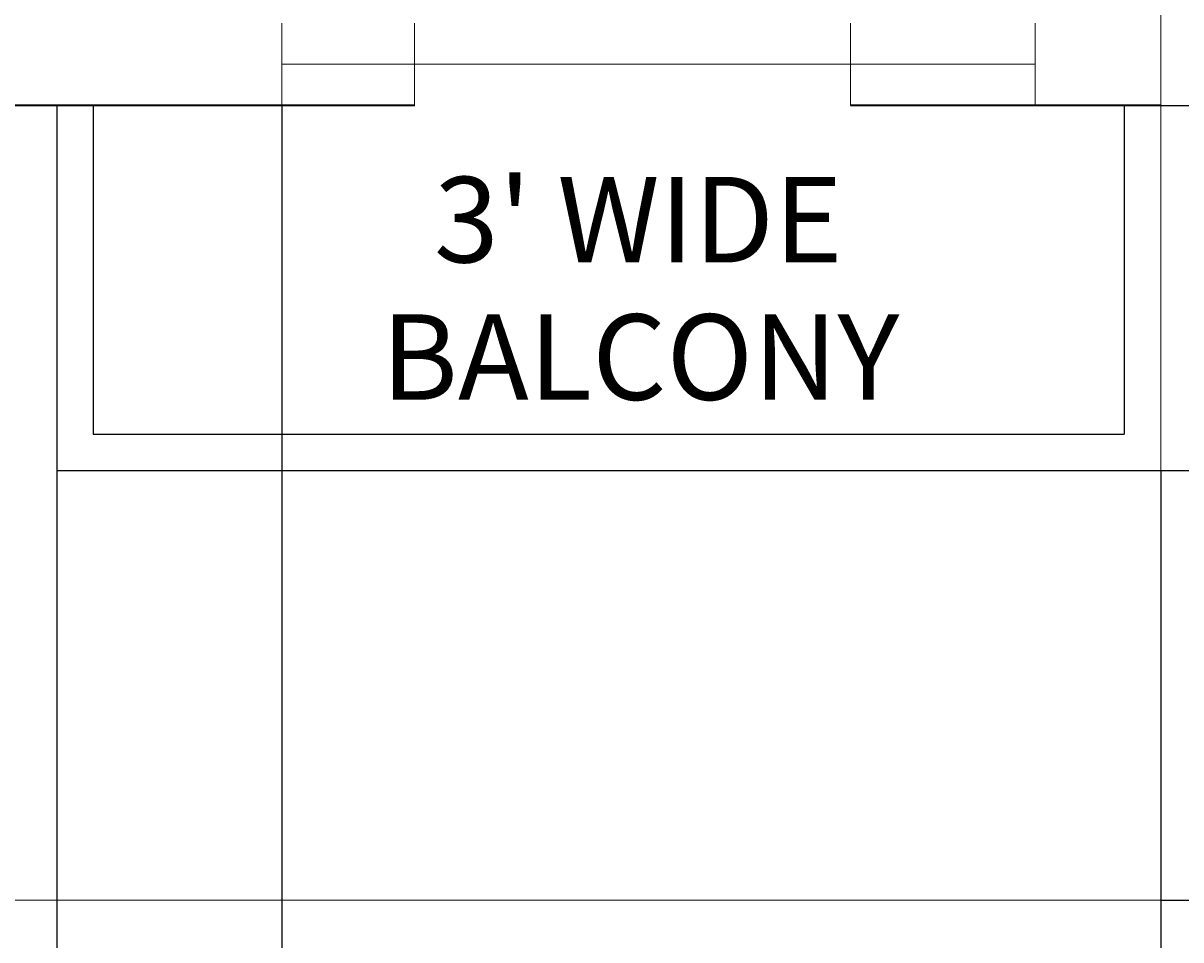
# Model space of a CAD drawing. Units: feet. Extents: x 2100 to 2836, y 2433 to 3396.
# Tile 4 of 12: x 2616 to 2743, y 2533 to 2634. Entities that reach past the tile are written whole.
import ezdxf

# ---------------------------------------------------------------- set-up
doc = ezdxf.new("R2010")
doc.units = ezdxf.units.FT
for name, color, linetype, lineweight in [('A-ANNO-DIMS', 2, 'Continuous', 18), ('A-AREA-IDEN', 7, 'Continuous', 18), ('A-DOOR', 3, 'Continuous', 18), ('A-FLOR-EDGE', 7, 'Continuous', 25), ('A-WALL', 7, 'Continuous', 35), ('C-PROP', 8, 'Continuous', 18)]:
    doc.layers.add(name, color=color, linetype=linetype, lineweight=lineweight)
doc.styles.get("Standard").update_dxf_attribs({"font": 'arial.ttf'})
doc.dimstyles.get("Standard").update_dxf_attribs({"dimtxt": 0.18, "dimasz": 0.18, "dimexe": 0.18, "dimexo": 0.0625, "dimgap": 0.09, "dimtad": 0, "dimtih": 1, "dimtoh": 1, "dimdec": 4, "dimzin": 0, "dimdsep": 46, "dimtxsty": 'Standard', "dimcen": 0.09, "dimadec": 0, "dimazin": 0, "dimtfac": 1, "dimtdec": 4, "dimtofl": 0, "dimtmove": 0, "dimatfit": 3, "dimfxl": 1, "dimtolj": 1, "dimtzin": 0, "dimarcsym": 0})

# ---------------------------------------------------------------- blocks, each defined once
blk = doc.blocks.new('DOOR-SLIDING-ENTRY')
for p, q in [((0, 9), (0, 0)), ((14.54, 9), (14.54, 0)), ((62.31, 9), (62.31, 0)), ((82.55, 9), (82.55, 0)), ((0, 4.5), (82.55, 4.5))]:
    blk.add_line(p, q)
blk = doc.blocks.new('*D42')
at = {"layer": 'A-ANNO-DIMS', "color": 0, "lineweight": -2, "transparency": 16777216}
for p, q in [((2521.95, 2537.69), (2521.95, 2433.01)), ((2740.95, 2537.69), (2740.95, 2433.01)), ((2522.13, 2433.19), (2631.16, 2433.19)), ((2740.77, 2433.19), (2631.74, 2433.19))]:
    blk.add_line(p, q, dxfattribs=at)
at = {"layer": 'A-ANNO-DIMS', "color": 0, "transparency": 16777216}
for points in [[(2522.13, 2433.22), (2522.13, 2433.16), (2521.95, 2433.19)], [(2740.77, 2433.22), (2740.77, 2433.16), (2740.95, 2433.19)]]:
    blk.add_solid(points, dxfattribs=at)
at = {"layer": 'Defpoints', "color": 0, "transparency": 16777216}
for p in [(2521.95, 2537.76), (2740.95, 2537.76), (2740.95, 2433.19)]:
    blk.add_point(p, dxfattribs=at)
at = {"layer": 'A-ANNO-DIMS', "color": 0, "transparency": 16777216, "insert": (2631.45, 2433.19), "char_height": 0.18, "attachment_point": 5}
blk.add_mtext('\\A1;219', dxfattribs=at)
blk = doc.blocks.new('*D56')
at = {"layer": 'A-ANNO-DIMS', "color": 0, "lineweight": -2, "transparency": 16777216}
for p, q in [((2741.01, 2584.8), (2835.49, 2584.8)), ((2835.31, 2584.62), (2835.31, 2561.46)), ((2835.31, 2537.94), (2835.31, 2561.1)), ((2741.01, 2537.76), (2835.49, 2537.76))]:
    blk.add_line(p, q, dxfattribs=at)
at = {"layer": 'A-ANNO-DIMS', "color": 0, "transparency": 16777216}
for points in [[(2835.28, 2584.62), (2835.34, 2584.62), (2835.31, 2584.8)], [(2835.28, 2537.94), (2835.34, 2537.94), (2835.31, 2537.76)]]:
    blk.add_solid(points, dxfattribs=at)
at = {"layer": 'Defpoints', "color": 0, "transparency": 16777216}
for p in [(2740.95, 2584.8), (2835.31, 2584.8), (2740.95, 2537.76)]:
    blk.add_point(p, dxfattribs=at)
at = {"layer": 'A-ANNO-DIMS', "color": 0, "transparency": 16777216, "insert": (2835.31, 2561.28), "char_height": 0.18, "attachment_point": 5}
blk.add_mtext('\\A1;47.05', dxfattribs=at)
blk = doc.blocks.new('*D57')
at = {"layer": 'A-ANNO-DIMS', "color": 0, "lineweight": -2, "transparency": 16777216}
for p, q in [((2741.01, 2662.65), (2835.49, 2662.65)), ((2835.31, 2662.47), (2835.31, 2643.91)), ((2835.31, 2624.98), (2835.31, 2643.54)), ((2741.01, 2624.8), (2835.49, 2624.8))]:
    blk.add_line(p, q, dxfattribs=at)
at = {"layer": 'A-ANNO-DIMS', "color": 0, "transparency": 16777216}
for points in [[(2835.28, 2662.47), (2835.34, 2662.47), (2835.31, 2662.65)], [(2835.28, 2624.98), (2835.34, 2624.98), (2835.31, 2624.8)]]:
    blk.add_solid(points, dxfattribs=at)
at = {"layer": 'Defpoints', "color": 0, "transparency": 16777216}
for p in [(2740.95, 2662.65), (2835.31, 2662.65), (2740.95, 2624.8)]:
    blk.add_point(p, dxfattribs=at)
at = {"layer": 'A-ANNO-DIMS', "color": 0, "transparency": 16777216, "insert": (2835.31, 2643.73), "char_height": 0.18, "attachment_point": 5}
blk.add_mtext('\\A1;37.845', dxfattribs=at)
blk = doc.blocks.new('*D65')
at = {"layer": 'A-ANNO-DIMS', "color": 0, "lineweight": -2, "transparency": 16777216}
for p, q in [((2619.95, 2624.74), (2619.95, 2433.01)), ((2644.63, 2624.74), (2644.63, 2433.01)), ((2620.13, 2433.19), (2631.83, 2433.19)), ((2644.45, 2433.19), (2632.76, 2433.19))]:
    blk.add_line(p, q, dxfattribs=at)
at = {"layer": 'A-ANNO-DIMS', "color": 0, "transparency": 16777216}
for points in [[(2620.13, 2433.22), (2620.13, 2433.16), (2619.95, 2433.19)], [(2644.45, 2433.22), (2644.45, 2433.16), (2644.63, 2433.19)]]:
    blk.add_solid(points, dxfattribs=at)
at = {"layer": 'Defpoints', "color": 0, "transparency": 16777216}
for p in [(2619.95, 2624.8), (2644.63, 2624.8), (2644.63, 2433.19)]:
    blk.add_point(p, dxfattribs=at)
at = {"layer": 'A-ANNO-DIMS', "color": 0, "transparency": 16777216, "insert": (2632.29, 2433.19), "char_height": 0.18, "attachment_point": 5}
blk.add_mtext('\\A1;24.686', dxfattribs=at)
blk = doc.blocks.new('*D66')
at = {"layer": 'A-ANNO-DIMS', "color": 0, "lineweight": -2, "transparency": 16777216}
for p, q in [((2619.95, 2584.74), (2619.95, 2433.01)), ((2740.95, 2584.74), (2740.95, 2433.01)), ((2620.13, 2433.19), (2680.18, 2433.19)), ((2740.77, 2433.19), (2680.71, 2433.19))]:
    blk.add_line(p, q, dxfattribs=at)
at = {"layer": 'A-ANNO-DIMS', "color": 0, "transparency": 16777216}
for points in [[(2620.13, 2433.22), (2620.13, 2433.16), (2619.95, 2433.19)], [(2740.77, 2433.22), (2740.77, 2433.16), (2740.95, 2433.19)]]:
    blk.add_solid(points, dxfattribs=at)
at = {"layer": 'Defpoints', "color": 0, "transparency": 16777216}
for p in [(2619.95, 2584.8), (2740.95, 2584.8), (2740.95, 2433.19)]:
    blk.add_point(p, dxfattribs=at)
at = {"layer": 'A-ANNO-DIMS', "color": 0, "transparency": 16777216, "insert": (2680.45, 2433.19), "char_height": 0.18, "attachment_point": 5}
blk.add_mtext('\\A1;121', dxfattribs=at)

msp = doc.modelspace()

# ---------------------------------------------------------------- linework, layer by layer
at = {"layer": 'A-FLOR-EDGE'}
for p, q in [((2619.9476, 2624.8031), (2619.9476, 2584.8031)), ((2623.9476, 2624.8031), (2623.9476, 2588.8031)), ((2736.9476, 2624.8031), (2736.9476, 2588.8031)), ((2623.9476, 2588.8031), (2736.9476, 2588.8031)), ((2619.9476, 2584.8031), (2740.9476, 2584.8031))]:
    msp.add_line(p, q, dxfattribs=at)
at = {"layer": 'A-WALL'}
for p, q in [((2659.1783, 2624.8031), (2521.9476, 2624.8031)), ((2740.9476, 2624.8031), (2706.9394, 2624.8031))]:
    msp.add_line(p, q, dxfattribs=at)
at = {"layer": 'C-PROP'}
for p in [(2740.9476, 2753.8031), (2521.9476, 2537.755)]:
    msp.add_line(p, (2740.9476, 2537.755), dxfattribs=at)

# ---------------------------------------------------------------- block references
at = {"layer": 'A-DOOR'}
msp.add_blockref('DOOR-SLIDING-ENTRY', (2644.6339, 2624.8031), dxfattribs=at)

# ---------------------------------------------------------------- texts
at = {"layer": 'A-AREA-IDEN'}
for s, p in [("3' WIDE ", (2661.2971, 2607.5988)), ('BALCONY', (2655.521, 2592.5502))]:
    msp.add_text(s, height=9.36783, dxfattribs=at).set_placement(p)

# ---------------------------------------------------------------- dimensions: what is measured, and where the dimension line sits
at = {"layer": 'A-ANNO-DIMS'}
for base, p1, p2, override, picture, middle in [((2835.3061, 2662.6479), (2740.9476, 2624.8031), (2740.9476, 2662.6479), {"dimdec": 3, "dimlfac": 1, "dimrnd": 0, "dimzin": 0, "dimdsep": 46, "dimlunit": 2}, '*D57', (2835.3061, 2643.7255)), ((2835.3061, 2584.8031), (2740.9476, 2537.755), (2740.9476, 2584.8031), {"dimdec": 2, "dimlfac": 1, "dimrnd": 0, "dimzin": 0, "dimdsep": 46, "dimlunit": 2}, '*D56', (2835.3061, 2561.2791))]:
    dim = msp.add_linear_dim(base=base, p1=p1, p2=p2, angle=90, dimstyle='Standard', override=override, dxfattribs=at)
    dim.commit()
    dim.dimension.update_dxf_attribs({"geometry": picture, "text_midpoint": middle})
for base, p1, p2, override, picture, middle in [((2644.6339, 2433.1873), (2619.9476, 2624.8031), (2644.6339, 2624.8031), {"dimdec": 3, "dimlfac": 1, "dimrnd": 0, "dimzin": 0, "dimdsep": 46, "dimlunit": 2}, '*D65', (2632.2907, 2433.1873)), ((2740.9476, 2433.1873), (2619.9476, 2584.8031), (2740.9476, 2584.8031), {"dimdec": 0, "dimlfac": 1, "dimrnd": 0, "dimzin": 0, "dimdsep": 46, "dimlunit": 2}, '*D66', (2680.4476, 2433.1873)), ((2740.9476, 2433.1873), (2521.9476, 2537.755), (2740.9476, 2537.755), {"dimdec": 0, "dimlfac": 1, "dimrnd": 0, "dimzin": 0, "dimdsep": 46, "dimlunit": 2}, '*D42', (2631.4476, 2433.1873))]:
    dim = msp.add_linear_dim(base=base, p1=p1, p2=p2, dimstyle='Standard', override=override, dxfattribs=at)
    dim.commit()
    dim.dimension.update_dxf_attribs({"geometry": picture, "text_midpoint": middle})

doc.saveas('drawing.dxf')
